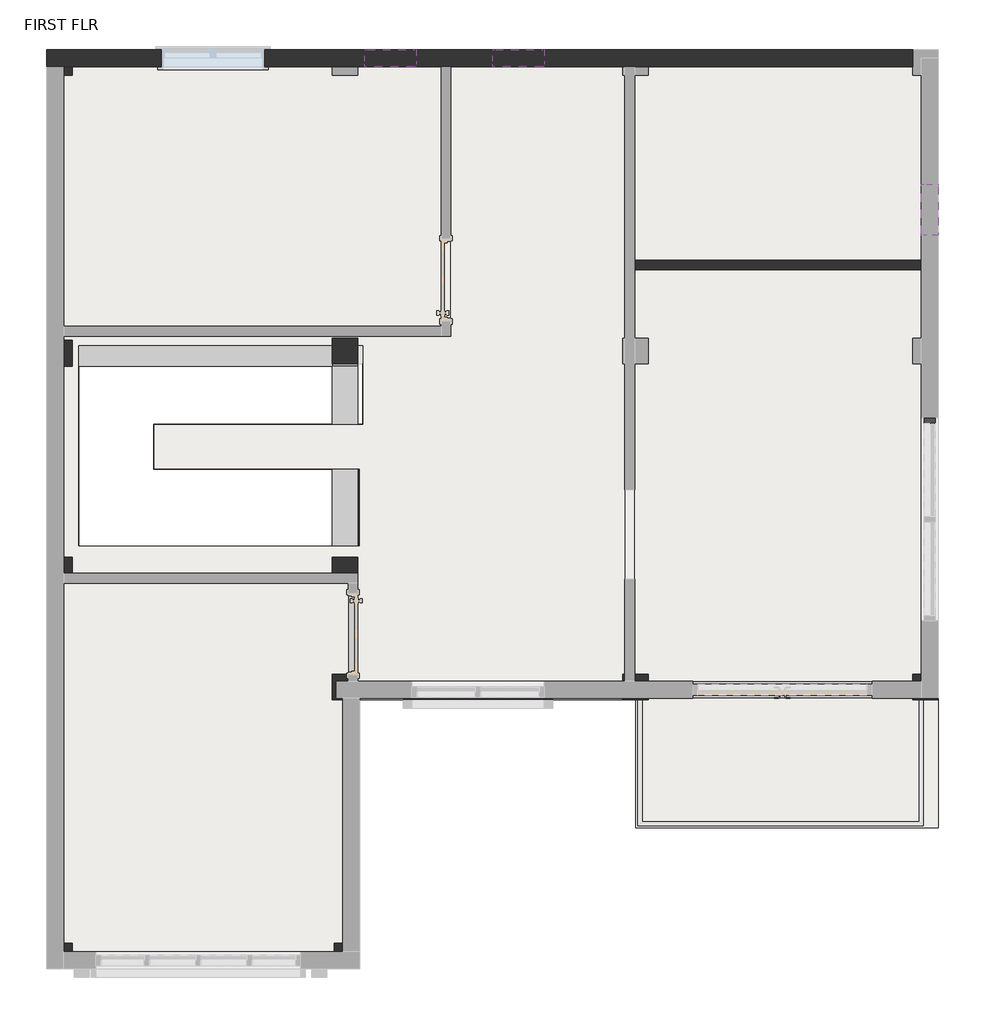
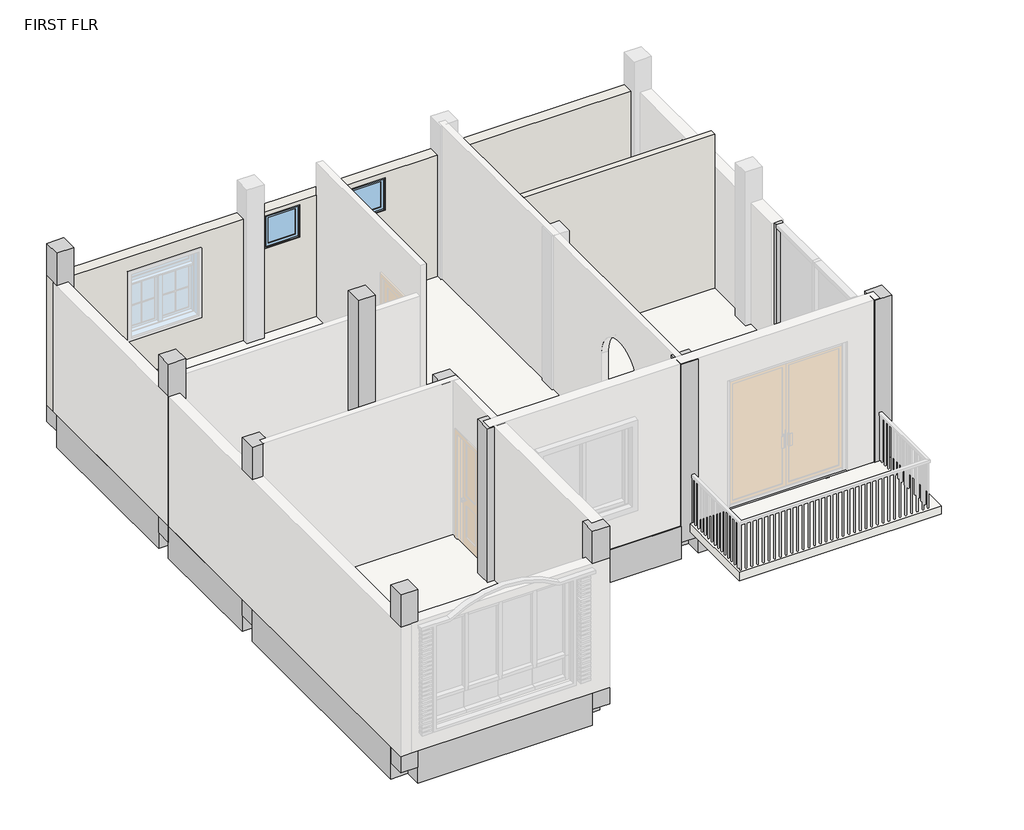
# One storey, part 2 of 3: 15 beams, 10 columns, 9 slabs, 3 windows, 2 walls, 1 member.
"""IFC4 building model written with IfcOpenShell, lengths in millimetres."""

from ifc_helpers import new_model, si_unit, frame, origin, place, context, project, spatial, polyline, outline, extrude, faceted_brep, transform, mapped, element, save
from components import member_5f9244a4, window_6846e476, window_347e55ac

model = new_model("IFC4")

# Units and contexts
model_context = context("Model", 3, world=origin())
ifc_project = project(units=[si_unit("LENGTHUNIT", "METRE", prefix="MILLI")], contexts=[model_context])

# Site, building, storey
site = spatial("IfcSite", under=ifc_project)
building = spatial("IfcBuilding", under=site)
storey = spatial("IfcBuildingStorey", under=building, Name="FIRST FLR", Elevation=3352.8)

# Beams
placement = place(None, origin())
element("IfcBeam", 1, ObjectType="Concrete-Rectangular Beam : 12 x 24", at=placement, inside=storey, context=model_context, shape_type="Brep", body=[
    faceted_brep([(-11643.8293601, -6018.4747117, 3352.8), (-11339.0293601, -6018.4747117, 3352.8), (-11339.0293601, -2868.8747117, 3352.8), (-11643.8293601, -2868.8747117, 3352.8), (-11643.8293601, -6018.4747117, 2743.2), (-11643.8293601, -6018.4747117, 3048.0), (-11643.8293601, -2868.8747117, 3048.0), (-11643.8293601, -2868.8747117, 2743.2), (-11339.0293601, -6018.4747117, 2743.2), (-11339.0293601, -2868.8747117, 2743.2), (-11339.0293601, -6018.4747117, 3048.0), (-11339.0293601, -2868.8747117, 3048.0)], [[[0, 1, 2, 3]], [[4, 5, 0, 3, 6, 7]], [[8, 4, 7, 9]], [[1, 10, 8, 9, 11, 2]], [[2, 11, 9, 7, 6, 3]], [[1, 0, 5, 4, 8, 10]]]),
])
element("IfcBeam", 2, ObjectType="Concrete-Rectangular Beam : 12 x 24", at=placement, inside=storey, context=model_context, shape_type="Brep", body=[
    faceted_brep([(-8251.5270642, -2868.8747117, 3352.8), (-8251.5270642, -2564.0747117, 3352.8), (-11339.0293601, -2564.0747117, 3352.8), (-11339.0293601, -2868.8747117, 3352.8), (-8251.5270642, -2868.8747117, 2743.2), (-8251.5270642, -2868.8747117, 3048.0), (-11339.0293601, -2868.8747117, 3048.0), (-11339.0293601, -2868.8747117, 2743.2), (-8251.5270642, -2564.0747117, 2743.2), (-11339.0293601, -2564.0747117, 2743.2), (-8251.5270642, -2564.0747117, 3048.0), (-11339.0293601, -2564.0747117, 3048.0)], [[[0, 1, 2, 3]], [[4, 5, 0, 3, 6, 7]], [[8, 4, 7, 9]], [[1, 10, 8, 9, 11, 2]], [[2, 11, 9, 7, 6, 3]], [[1, 0, 5, 4, 8, 10]]]),
])
element("IfcBeam", 3, ObjectType="Concrete-Rectangular Beam : 12 x 24", at=placement, inside=storey, context=model_context, shape_type="Brep", body=[
    faceted_brep([(-7946.7270642, -2868.8747117, 3352.8), (-8251.5270642, -2868.8747117, 3352.8), (-8251.5270642, -5993.0747117, 3352.8), (-7946.7270642, -5993.0747117, 3352.8), (-8251.5270642, -2868.8747117, 3048.0), (-8251.5270642, -2868.8747117, 2743.2), (-8251.5270642, -5993.0747117, 2743.2), (-8251.5270642, -5993.0747117, 3048.0), (-7946.7270642, -2868.8747117, 2743.2), (-7946.7270642, -5993.0747117, 2743.2), (-7946.7270642, -2868.8747117, 3048.0), (-7946.7270642, -5993.0747117, 3048.0)], [[[0, 1, 2, 3]], [[1, 4, 5, 6, 7, 2]], [[5, 8, 9, 6]], [[8, 10, 0, 3, 11, 9]], [[0, 10, 8, 5, 4, 1]], [[3, 2, 7, 6, 9, 11]]]),
    faceted_brep([(-7946.7270642, -6323.2747117, 3352.8), (-8251.5270642, -6323.2747117, 3352.8), (-8251.5270642, -6323.2747117, 2743.2), (-7946.7270642, -6323.2747117, 2743.2), (-8251.5270642, -6297.8747117, 3352.8), (-7946.7270642, -6297.8747117, 3352.8), (-7946.7270642, -6297.8747117, 3048.0), (-7946.7270642, -6297.8747117, 2743.2), (-8251.5270642, -6297.8747117, 2743.2), (-8251.5270642, -6297.8747117, 3048.0)], [[[0, 1, 2, 3]], [[4, 5, 6, 7, 8, 9]], [[1, 0, 5, 4]], [[2, 1, 4, 9, 8]], [[3, 2, 8, 7]], [[0, 3, 7, 6, 5]]]),
])
element("IfcBeam", 4, ObjectType="Concrete-Rectangular Beam : 12 x 24", at=placement, inside=storey, context=model_context, shape_type="Brep", body=[
    faceted_brep([(-1351.9658472, -9984.0050402, 3352.8), (-1047.1658472, -9984.0050402, 3352.8), (-1047.1658472, -6297.8747117, 3352.8), (-1351.9658472, -6297.8747117, 3352.8), (-1351.9658472, -9984.0050402, 2743.2), (-1351.9658472, -9984.0050402, 3048.0), (-1351.9658472, -6297.8747117, 3048.0), (-1351.9658472, -6297.8747117, 2743.2), (-1047.1658472, -9984.0050402, 2743.2), (-1047.1658472, -6297.8747117, 2743.2), (-1047.1658472, -9984.0050402, 3048.0), (-1047.1658472, -6297.8747117, 3048.0)], [[[0, 1, 2, 3]], [[4, 5, 0, 3, 6, 7]], [[8, 4, 7, 9]], [[1, 10, 8, 9, 11, 2]], [[2, 11, 9, 7, 6, 3]], [[1, 0, 5, 4, 8, 10]]]),
])
element("IfcBeam", 5, ObjectType="Concrete-Rectangular Beam : 12 x 24", at=placement, inside=storey, context=model_context, shape_type="Brep", body=[
    faceted_brep([(-4492.3270642, -9984.0050402, 3352.8), (-4492.3270642, -10288.8050402, 3352.8), (-1351.9658472, -10288.8050402, 3352.8), (-1351.9658472, -9984.0050402, 3352.8), (-4492.3270642, -9984.0050402, 2743.2), (-4492.3270642, -9984.0050402, 3048.0), (-1351.9658472, -9984.0050402, 3048.0), (-1351.9658472, -9984.0050402, 2743.2), (-4492.3270642, -10288.8050402, 2743.2), (-1351.9658472, -10288.8050402, 2743.2), (-4492.3270642, -10288.8050402, 3048.0), (-1351.9658472, -10288.8050402, 3048.0)], [[[0, 1, 2, 3]], [[4, 5, 0, 3, 6, 7]], [[8, 4, 7, 9]], [[1, 10, 8, 9, 11, 2]], [[1, 0, 5, 4, 8, 10]], [[2, 11, 9, 7, 6, 3]]]),
])
element("IfcBeam", 6, ObjectType="Concrete-Rectangular Beam : 12 x 24", at=placement, inside=storey, context=model_context, shape_type="Brep", body=[
    faceted_brep([(-7946.7270642, -9984.0050402, 3352.8), (-7946.7270642, -10288.8050402, 3352.8), (-7921.3270642, -10288.8050402, 3352.8), (-4797.1270642, -10288.8050402, 3352.8), (-4797.1270642, -9984.0050402, 3352.8), (-4801.7464557, -9984.0050402, 3352.8), (-7942.1076727, -9984.0050402, 3352.8), (-7946.7270642, -9984.0050402, 2743.2), (-7946.7270642, -9984.0050402, 3048.0), (-4797.1270642, -9984.0050402, 3048.0), (-4797.1270642, -9984.0050402, 2743.2), (-7946.7270642, -10288.8050402, 2743.2), (-4797.1270642, -10288.8050402, 2743.2), (-7921.3270642, -10288.8050402, 2743.2), (-7946.7270642, -10288.8050402, 3048.0), (-4797.1270642, -10288.8050402, 3048.0)], [[[0, 1, 2, 3, 4, 5, 6]], [[7, 8, 0, 6, 5, 4, 9, 10]], [[11, 7, 10, 12, 13]], [[1, 14, 11, 13, 12, 15, 3, 2]], [[1, 0, 8, 7, 11, 14]], [[3, 15, 12, 10, 9, 4]]]),
])
element("IfcBeam", 7, ObjectType="Concrete-Rectangular Beam : 12 x 24", at=placement, inside=storey, context=model_context, shape_type="Brep", body=[
    faceted_brep([(-7946.7270642, -9984.0050402, 3352.8), (-7946.7270642, -8902.7373391, 3352.8), (-8226.1270642, -8902.7373391, 3352.8), (-8226.1270642, -9984.0050402, 3352.8), (-7946.7270642, -9984.0050402, 3048.0), (-7946.7270642, -9984.0050402, 2743.2), (-7946.7270642, -8902.7373391, 2743.2), (-7946.7270642, -8902.7373391, 3048.0), (-8251.5270642, -9984.0050402, 2743.2), (-8251.5270642, -8902.7373391, 2743.2), (-8251.5270642, -9984.0050402, 3048.0), (-8251.5270642, -8902.7373391, 3048.0), (-8226.1270642, -8902.7373391, 3048.0), (-8226.1270642, -9984.0050402, 3048.0)], [[[0, 1, 2, 3]], [[1, 0, 4, 5, 6, 7]], [[6, 5, 8, 9]], [[9, 8, 10, 11]], [[1, 7, 6, 9, 11, 12, 2]], [[8, 5, 4, 0, 3, 13, 10]], [[13, 12, 11, 10]], [[12, 13, 3, 2]]]),
])
element("IfcBeam", 8, ObjectType="Concrete-Rectangular Beam : 12 x 24", at=placement, inside=storey, context=model_context, shape_type="Brep", body=[
    faceted_brep([(-8251.5270642, -8597.9373391, 3352.8), (-7946.7270642, -8597.9373391, 3352.8), (-7946.7270642, -6323.2747117, 3352.8), (-8251.5270642, -6323.2747117, 3352.8), (-8251.5270642, -7013.8396616, 3352.8), (-8251.5270642, -7547.2396616, 3352.8), (-8251.5270642, -8461.6396616, 3352.8), (-7946.7270642, -8597.9373391, 3048.0), (-7946.7270642, -8597.9373391, 2743.2), (-7946.7270642, -6323.2747117, 2743.2), (-8251.5270642, -8597.9373391, 2743.2), (-8251.5270642, -6323.2747117, 2743.2), (-8251.5270642, -8597.9373391, 3048.0)], [[[0, 1, 2, 3, 4, 5, 6]], [[1, 7, 8, 9, 2]], [[8, 10, 11, 9]], [[10, 12, 0, 6, 5, 4, 3, 11]], [[0, 12, 10, 8, 7, 1]], [[3, 2, 9, 11]]]),
])
element("IfcBeam", 9, ObjectType="Concrete-Rectangular Beam : 12 x 24", at=placement, inside=storey, context=model_context, shape_type="Brep", body=[
    faceted_brep([(-11339.0293601, -8597.9373391, 3352.8), (-11339.0293601, -8902.7373391, 3352.8), (-8251.5270642, -8902.7373391, 3352.8), (-8251.5270642, -8597.9373391, 3352.8), (-11339.0293601, -8597.9373391, 2743.2), (-11339.0293601, -8597.9373391, 3048.0), (-8251.5270642, -8597.9373391, 3048.0), (-8251.5270642, -8597.9373391, 2743.2), (-11339.0293601, -8902.7373391, 2743.2), (-8251.5270642, -8902.7373391, 2743.2), (-11339.0293601, -8902.7373391, 3048.0), (-8251.5270642, -8902.7373391, 3048.0)], [[[0, 1, 2, 3]], [[4, 5, 0, 3, 6, 7]], [[8, 4, 7, 9]], [[1, 10, 8, 9, 11, 2]], [[1, 0, 5, 4, 8, 10]], [[2, 11, 9, 7, 6, 3]]]),
])
element("IfcBeam", 10, ObjectType="Concrete-Rectangular Beam : 12 x 24", at=placement, inside=storey, context=model_context, shape_type="Brep", body=[
    faceted_brep([(-11339.0293601, -6323.2747117, 3352.8), (-11643.8293601, -6323.2747117, 3352.8), (-11643.8293601, -8597.9373391, 3352.8), (-11339.0293601, -8597.9373391, 3352.8), (-11339.0293601, -6323.2747117, 2743.2), (-11339.0293601, -6323.2747117, 3048.0), (-11339.0293601, -8597.9373391, 3048.0), (-11339.0293601, -8597.9373391, 2743.2), (-11643.8293601, -6323.2747117, 2743.2), (-11643.8293601, -8597.9373391, 2743.2), (-11643.8293601, -6323.2747117, 3048.0), (-11643.8293601, -8597.9373391, 3048.0)], [[[0, 1, 2, 3]], [[4, 5, 0, 3, 6, 7]], [[8, 4, 7, 9]], [[1, 10, 8, 9, 11, 2]], [[1, 0, 5, 4, 8, 10]], [[2, 11, 9, 7, 6, 3]]]),
])
element("IfcBeam", 11, ObjectType="Concrete-Rectangular Beam : 12 x 24", at=placement, inside=storey, context=model_context, shape_type="Brep", body=[
    faceted_brep([(-8251.5270642, -6018.4747117, 3352.8), (-8251.5270642, -6297.8747117, 3352.8), (-8251.5270642, -6323.2747117, 3352.8), (-8251.5270642, -6323.2747117, 2743.2), (-8251.5270642, -6297.8747117, 2743.2), (-8251.5270642, -6018.4747117, 2743.2), (-8251.5270642, -6018.4747117, 3048.0), (-11339.0293601, -6018.4747117, 3352.8), (-11339.0293601, -6323.2747117, 3352.8), (-11264.7236584, -6323.2747117, 3352.8), (-11339.0293601, -6323.2747117, 3048.0), (-11339.0293601, -6323.2747117, 2743.2), (-11339.0293601, -6018.4747117, 2743.2), (-11339.0293601, -6018.4747117, 3048.0)], [[[0, 1, 2, 3, 4, 5, 6]], [[2, 1, 0, 7, 8, 9]], [[3, 2, 9, 8, 10, 11]], [[5, 4, 3, 11, 12]], [[0, 6, 5, 12, 13, 7]], [[7, 13, 12, 11, 10, 8]]]),
])
element("IfcBeam", 12, ObjectType="Concrete-Rectangular Beam : 12 x 24", at=placement, inside=storey, context=model_context, shape_type="Brep", body=[
    faceted_brep([(-4492.3270642, -6297.8747117, 3352.8), (-4797.1270642, -6297.8747117, 3352.8), (-4797.1270642, -9984.0050402, 3352.8), (-4492.3270642, -9984.0050402, 3352.8), (-4492.3270642, -6297.8747117, 2743.2), (-4492.3270642, -6297.8747117, 3048.0), (-4492.3270642, -9984.0050402, 3048.0), (-4492.3270642, -9984.0050402, 2743.2), (-4797.1270642, -6297.8747117, 2743.2), (-4797.1270642, -9984.0050402, 2743.2), (-4797.1270642, -6297.8747117, 3048.0), (-4797.1270642, -9984.0050402, 3048.0)], [[[0, 1, 2, 3]], [[4, 5, 0, 3, 6, 7]], [[8, 4, 7, 9]], [[1, 10, 8, 9, 11, 2]], [[1, 0, 5, 4, 8, 10]], [[2, 11, 9, 7, 6, 3]]]),
])
element("IfcBeam", 13, ObjectType="Concrete-Rectangular Beam : 12 x 24", at=placement, inside=storey, context=model_context, shape_type="Brep", body=[
    faceted_brep([(-11339.0293601, -8902.7373391, 3352.8), (-11643.8293601, -8902.7373391, 3352.8), (-11643.8293601, -13183.002305, 3352.8), (-11339.0293601, -13183.002305, 3352.8), (-11339.0293601, -8902.7373391, 2743.2), (-11339.0293601, -8902.7373391, 3048.0), (-11339.0293601, -13183.002305, 3048.0), (-11339.0293601, -13183.002305, 2743.2), (-11643.8293601, -8902.7373391, 2743.2), (-11643.8293601, -13183.002305, 2743.2), (-11643.8293601, -8902.7373391, 3048.0), (-11643.8293601, -13183.002305, 3048.0)], [[[0, 1, 2, 3]], [[4, 5, 0, 3, 6, 7]], [[8, 4, 7, 9]], [[1, 10, 8, 9, 11, 2]], [[1, 0, 5, 4, 8, 10]], [[2, 11, 9, 7, 6, 3]]]),
])
element("IfcBeam", 14, ObjectType="Concrete-Rectangular Beam : 12 x 24", at=placement, inside=storey, context=model_context, shape_type="Brep", body=[
    faceted_brep([(-7921.3270642, -10288.8050402, 3352.8), (-7946.7270642, -10288.8050402, 3352.8), (-8226.1270642, -10288.8050402, 3352.8), (-8226.1270642, -13183.002305, 3352.8), (-7921.3270642, -13183.002305, 3352.8), (-8226.1270642, -10288.8050402, 3048.0), (-8226.1270642, -10288.8050402, 2743.2), (-8226.1270642, -13183.002305, 2743.2), (-8226.1270642, -13183.002305, 3048.0), (-7946.7270642, -10288.8050402, 2743.2), (-7921.3270642, -10288.8050402, 2743.2), (-7921.3270642, -13183.002305, 2743.2), (-7921.3270642, -13183.002305, 3048.0)], [[[0, 1, 2, 3, 4]], [[2, 5, 6, 7, 8, 3]], [[6, 9, 10, 11, 7]], [[10, 0, 4, 12, 11]], [[0, 10, 9, 6, 5, 2, 1]], [[4, 3, 8, 7, 11, 12]]]),
])
element("IfcBeam", 15, ObjectType="Concrete-Rectangular Beam : 12 x 24", at=placement, inside=storey, context=model_context, shape_type="Brep", body=[
    faceted_brep([(-11339.0293601, -13183.002305, 3352.8), (-11339.0293601, -13487.802305, 3352.8), (-8226.1270642, -13487.802305, 3352.8), (-8226.1270642, -13183.002305, 3352.8), (-11339.0293601, -13183.002305, 2743.2), (-11339.0293601, -13183.002305, 3048.0), (-8226.1270642, -13183.002305, 3048.0), (-8226.1270642, -13183.002305, 2743.2), (-11339.0293601, -13487.802305, 2743.2), (-8226.1270642, -13487.802305, 2743.2), (-11339.0293601, -13487.802305, 3048.0), (-8226.1270642, -13487.802305, 3048.0)], [[[0, 1, 2, 3]], [[4, 5, 0, 3, 6, 7]], [[8, 4, 7, 9]], [[1, 10, 8, 9, 11, 2]], [[2, 11, 9, 7, 6, 3]], [[1, 0, 5, 4, 8, 10]]]),
])

# Columns
element("IfcColumn", 16, ObjectType="Concrete-Rectangular-Column : 12\" X 12\" COLUMN", at=placement, inside=storey, context=model_context, shape_type="Brep", body=[
    faceted_brep([(-11339.0293601, -2564.0747117, 3048.0), (-11339.0293601, -2868.8747117, 3048.0), (-11643.8293601, -2868.8747117, 3048.0), (-11643.8293601, -2564.0747117, 3048.0), (-11339.0293601, -2564.0747117, 6400.8), (-11339.0293601, -2868.8747117, 6400.8), (-11339.0293601, -2868.8747117, 3352.8), (-11339.0293601, -2564.0747117, 3352.8), (-11643.8293601, -2868.8747117, 6400.8), (-11643.8293601, -2868.8747117, 3352.8), (-11643.8293601, -2564.0747117, 6400.8)], [[[0, 1, 2, 3]], [[4, 5, 6, 1, 0, 7]], [[5, 8, 9, 2, 1, 6]], [[8, 10, 3, 2, 9]], [[10, 4, 7, 0, 3]], [[4, 10, 8, 5]]]),
])
element("IfcColumn", 17, ObjectType="Concrete-Rectangular-Column : 12\" X 12\" COLUMN", at=placement, inside=storey, context=model_context, shape_type="Brep", body=[
    faceted_brep([(-7946.7270642, -5993.0747117, 3048.0), (-7946.7270642, -6297.8747117, 3048.0), (-8251.5270642, -6297.8747117, 3048.0), (-8251.5270642, -6018.4747117, 3048.0), (-8251.5270642, -5993.0747117, 3048.0), (-7946.7270642, -5993.0747117, 6400.8), (-7946.7270642, -6297.8747117, 6400.8), (-7946.7270642, -6297.8747117, 3352.8), (-7946.7270642, -5993.0747117, 3352.8), (-8251.5270642, -6297.8747117, 6400.8), (-8251.5270642, -6297.8747117, 3352.8), (-8251.5270642, -5993.0747117, 6400.8), (-8251.5270642, -5993.0747117, 3352.8)], [[[0, 1, 2, 3, 4]], [[5, 6, 7, 1, 0, 8]], [[6, 9, 10, 2, 1, 7]], [[9, 11, 12, 4, 3, 2, 10]], [[11, 5, 8, 0, 4, 12]], [[5, 11, 9, 6]]]),
])
element("IfcColumn", 18, ObjectType="Concrete-Rectangular-Column : 12\" X 12\" COLUMN", at=placement, inside=storey, context=model_context, shape_type="Brep", body=[
    faceted_brep([(-11339.0293601, -6018.4747117, 3048.0), (-11339.0293601, -6323.2747117, 3048.0), (-11643.8293601, -6323.2747117, 3048.0), (-11643.8293601, -6018.4747117, 3048.0), (-11339.0293601, -6018.4747117, 6400.8), (-11339.0293601, -6323.2747117, 6400.8), (-11339.0293601, -6323.2747117, 3352.8), (-11339.0293601, -6018.4747117, 3352.8), (-11643.8293601, -6323.2747117, 6400.8), (-11643.8293601, -6323.2747117, 3352.8), (-11643.8293601, -6018.4747117, 6400.8), (-11643.8293601, -6018.4747117, 3352.8)], [[[0, 1, 2, 3]], [[4, 5, 6, 1, 0, 7]], [[5, 8, 9, 2, 1, 6]], [[8, 10, 11, 3, 2, 9]], [[10, 4, 7, 0, 3, 11]], [[4, 10, 8, 5]]]),
])
element("IfcColumn", 19, ObjectType="Concrete-Rectangular-Column : 12\" X 12\" COLUMN", at=placement, inside=storey, context=model_context, shape_type="Brep", body=[
    faceted_brep([(-11339.0293601, -8597.9373391, 3048.0), (-11339.0293601, -8902.7373391, 3048.0), (-11643.8293601, -8902.7373391, 3048.0), (-11643.8293601, -8597.9373391, 3048.0), (-11339.0293601, -8597.9373391, 6400.8), (-11339.0293601, -8902.7373391, 6400.8), (-11339.0293601, -8902.7373391, 3352.8), (-11339.0293601, -8597.9373391, 3352.8), (-11643.8293601, -8902.7373391, 6400.8), (-11643.8293601, -8902.7373391, 3352.8), (-11643.8293601, -8597.9373391, 6400.8), (-11643.8293601, -8597.9373391, 3352.8)], [[[0, 1, 2, 3]], [[4, 5, 6, 1, 0, 7]], [[5, 8, 9, 2, 1, 6]], [[8, 10, 11, 3, 2, 9]], [[10, 4, 7, 0, 3, 11]], [[4, 10, 8, 5]]]),
])
element("IfcColumn", 20, ObjectType="Concrete-Rectangular-Column : 12\" X 12\" COLUMN", at=placement, inside=storey, context=model_context, shape_type="Brep", body=[
    faceted_brep([(-7946.7270642, -8597.9373391, 3048.0), (-7946.7270642, -8902.7373391, 3048.0), (-8251.5270642, -8902.7373391, 3048.0), (-8251.5270642, -8597.9373391, 3048.0), (-7946.7270642, -8597.9373391, 6400.8), (-7946.7270642, -8902.7373391, 6400.8), (-7946.7270642, -8902.7373391, 3352.8), (-7946.7270642, -8597.9373391, 3352.8), (-8251.5270642, -8902.7373391, 6400.8), (-8251.5270642, -8902.7373391, 3352.8), (-8251.5270642, -8597.9373391, 6400.8), (-8251.5270642, -8597.9373391, 3352.8)], [[[0, 1, 2, 3]], [[4, 5, 6, 1, 0, 7]], [[5, 8, 9, 2, 1, 6]], [[8, 10, 11, 3, 2, 9]], [[10, 4, 7, 0, 3, 11]], [[4, 10, 8, 5]]]),
])
element("IfcColumn", 21, ObjectType="Concrete-Rectangular-Column : 12\" X 12\" COLUMN", at=placement, inside=storey, context=model_context, shape_type="Brep", body=[
    faceted_brep([(-7921.3270642, -13183.002305, 3048.0), (-7921.3270642, -13487.802305, 3048.0), (-8226.1270642, -13487.802305, 3048.0), (-8226.1270642, -13183.002305, 3048.0), (-7921.3270642, -13183.002305, 6400.8), (-7921.3270642, -13487.802305, 6400.8), (-7921.3270642, -13183.002305, 3352.8), (-8226.1270642, -13487.802305, 6400.8), (-8226.1270642, -13487.802305, 3352.8), (-8226.1270642, -13183.002305, 6400.8), (-8226.1270642, -13183.002305, 3352.8)], [[[0, 1, 2, 3]], [[4, 5, 1, 0, 6]], [[5, 7, 8, 2, 1]], [[7, 9, 10, 3, 2, 8]], [[9, 4, 6, 0, 3, 10]], [[4, 9, 7, 5]]]),
])
element("IfcColumn", 22, ObjectType="Concrete-Rectangular-Column : 12\" X 12\" COLUMN", at=placement, inside=storey, context=model_context, shape_type="Brep", body=[
    faceted_brep([(-11339.0293601, -13183.002305, 3048.0), (-11339.0293601, -13487.802305, 3048.0), (-11643.8293601, -13487.802305, 3048.0), (-11643.8293601, -13183.002305, 3048.0), (-11339.0293601, -13183.002305, 6400.8), (-11339.0293601, -13487.802305, 6400.8), (-11339.0293601, -13487.802305, 3352.8), (-11339.0293601, -13183.002305, 3352.8), (-11643.8293601, -13487.802305, 6400.8), (-11643.8293601, -13183.002305, 6400.8), (-11643.8293601, -13183.002305, 3352.8)], [[[0, 1, 2, 3]], [[4, 5, 6, 1, 0, 7]], [[5, 8, 2, 1, 6]], [[8, 9, 10, 3, 2]], [[9, 4, 7, 0, 3, 10]], [[4, 9, 8, 5]]]),
])
element("IfcColumn", 23, ObjectType="Concrete-Rectangular-Column : 12\" X 12\" COLUMN", at=placement, inside=storey, context=model_context, shape_type="Brep", body=[
    faceted_brep([(-7946.7270642, -9984.0050402, 3048.0), (-7946.7270642, -10288.8050402, 3048.0), (-8226.1270642, -10288.8050402, 3048.0), (-8226.1270642, -9984.0050402, 3048.0), (-7946.7270642, -9984.0050402, 3352.8), (-7946.7270642, -9984.0050402, 6400.8), (-7946.7270642, -10288.8050402, 6400.8), (-7946.7270642, -10288.8050402, 3352.8), (-8251.5270642, -10288.8050402, 6400.8), (-8251.5270642, -10288.8050402, 3352.8), (-8226.1270642, -10288.8050402, 3352.8), (-8251.5270642, -9984.0050402, 6400.8), (-8251.5270642, -9984.0050402, 3352.8), (-8226.1270642, -9984.0050402, 3352.8)], [[[0, 1, 2, 3]], [[1, 0, 4, 5, 6, 7]], [[1, 7, 6, 8, 9, 10, 2]], [[8, 11, 12, 9]], [[5, 4, 0, 3, 13, 12, 11]], [[6, 5, 11, 8]], [[13, 10, 9, 12]], [[10, 13, 3, 2]]]),
])
element("IfcColumn", 24, ObjectType="Concrete-Rectangular-Column : 12\" X 12\" COLUMN", at=placement, inside=storey, context=model_context, shape_type="Brep", body=[
    faceted_brep([(-4492.3270642, -9984.0050402, 3048.0), (-4492.3270642, -10288.8050402, 3048.0), (-4797.1270642, -10288.8050402, 3048.0), (-4797.1270642, -9984.0050402, 3048.0), (-4492.3270642, -9984.0050402, 6400.8), (-4492.3270642, -10288.8050402, 6400.8), (-4492.3270642, -10288.8050402, 3352.8), (-4492.3270642, -9984.0050402, 3352.8), (-4797.1270642, -10288.8050402, 6400.8), (-4797.1270642, -10288.8050402, 3352.8), (-4797.1270642, -9984.0050402, 6400.8), (-4797.1270642, -9984.0050402, 3352.8)], [[[0, 1, 2, 3]], [[4, 5, 6, 1, 0, 7]], [[5, 8, 9, 2, 1, 6]], [[8, 10, 11, 3, 2, 9]], [[10, 4, 7, 0, 3, 11]], [[4, 10, 8, 5]]]),
])
element("IfcColumn", 25, ObjectType="Concrete-Rectangular-Column : 12\" X 12\" COLUMN", at=placement, inside=storey, context=model_context, shape_type="Brep", body=[
    faceted_brep([(-1047.1658472, -9984.0050402, 3048.0), (-1047.1658472, -10288.8050402, 3048.0), (-1351.9658472, -10288.8050402, 3048.0), (-1351.9658472, -9984.0050402, 3048.0), (-1047.1658472, -9984.0050402, 6400.8), (-1047.1658472, -10288.8050402, 6400.8), (-1047.1658472, -9984.0050402, 3352.8), (-1351.9658472, -10288.8050402, 6400.8), (-1351.9658472, -10288.8050402, 3352.8), (-1351.9658472, -9984.0050402, 6400.8), (-1351.9658472, -9984.0050402, 3352.8)], [[[0, 1, 2, 3]], [[4, 5, 1, 0, 6]], [[5, 7, 8, 2, 1]], [[7, 9, 10, 3, 2, 8]], [[9, 4, 6, 0, 3, 10]], [[4, 9, 7, 5]]]),
])

# Member
member_shape = member_5f9244a4(model_context)
element("IfcMember", 26, ObjectType="Rectangular Mullion : 2.5\" x 5\" rectangular", at=placement, inside=storey, context=model_context, shape_type="MappedRepresentation", body=[
    mapped(member_shape, transform((-1148.7658472, -6939.2247117, 5791.2), x_axis=(0.0, 1.0, 0.0), y_axis=(-1.0, 0.0, 0.0), z_axis=(0.0, 0.0, 1.0))),
])

# Slabs
element("IfcSlab", 27, ObjectType="FLOORING 6\"", at=placement, inside=storey, context=model_context, shape_type="SweptSolid", body=[
    extrude(outline(polyline([(-4644.7270642, -10271.3896616), (-1047.1658472, -10271.3896616), (-1047.1658472, -11812.34549), (-4644.7270642, -11812.34549), (-4644.7270642, -10271.3896616)])), frame((0.0, 0.0, 3200.4), z_axis=(0.0, 0.0, 1.0), x_axis=(1.0, 0.0, 0.0)), (0.0, 0.0, 1.0), 152.4),
])
element("IfcSlab", 28, ObjectType="FLOORING 6\"", at=placement, inside=storey, context=model_context, shape_type="SweptSolid", body=[
    extrude(outline(polyline([(-6956.1270642, -2767.2747117), (-6956.1270642, -5851.7896616), (-11442.5236584, -5851.7896616), (-11442.5236584, -2767.2747117), (-6956.1270642, -2767.2747117)])), frame((0.0, 0.0, 3352.8), z_axis=(0.0, 0.0, 1.0), x_axis=(1.0, 0.0, 0.0)), (0.0, 0.0, 1.0), 152.4),
    extrude(outline(polyline([(-1250.3658472, -2767.2747117), (-1250.3658472, -5064.3896616), (-4657.4270642, -5064.3896616), (-4657.4270642, -2767.2747117), (-1250.3658472, -2767.2747117)])), frame((0.0, 0.0, 3352.8), z_axis=(0.0, 0.0, 1.0), x_axis=(1.0, 0.0, 0.0)), (0.0, 0.0, 1.0), 152.4),
    extrude(outline(polyline([(-4657.4270642, -10068.1896616), (-4657.4270642, -5178.6896616), (-1250.3658472, -5178.6896616), (-1250.3658472, -10068.1896616), (-4657.4270642, -10068.1896616)])), frame((0.0, 0.0, 3352.8), z_axis=(0.0, 0.0, 1.0), x_axis=(1.0, 0.0, 0.0)), (0.0, 0.0, 1.0), 152.4),
    extrude(outline(polyline([(-8061.0270642, -8902.7373391), (-8061.0270642, -10068.1896616), (-8200.7270642, -10068.1896616), (-8200.7270642, -10271.3896616), (-8124.5270642, -10271.3896616), (-8124.5270642, -13284.602305), (-11442.5236584, -13284.602305), (-11442.5236584, -8902.7373391), (-8061.0270642, -8902.7373391)])), frame((0.0, 0.0, 3352.8), z_axis=(0.0, 0.0, 1.0), x_axis=(1.0, 0.0, 0.0)), (0.0, 0.0, 1.0), 152.4),
    extrude(outline(polyline([(-6841.8270642, -5966.0896616), (-6841.8270642, -2767.2747117), (-4771.7270642, -2767.2747117), (-4771.7270642, -10068.1896616), (-7946.7270642, -10068.1896616), (-7946.7270642, -8788.4373391), (-11442.5236584, -8788.4373391), (-11442.5236584, -5966.0896616), (-6841.8270642, -5966.0896616)]), holes=[polyline([(-11264.7236584, -6080.3896616), (-11264.7236584, -8461.6396616), (-7930.9736584, -8461.6396616), (-7930.9736584, -7547.2396616), (-10369.3736584, -7547.2396616), (-10369.3736584, -7013.8396616), (-7889.5770642, -7013.8396616), (-7889.5770642, -6080.3896616), (-11264.7236584, -6080.3896616)])]), frame((0.0, 0.0, 3352.8), z_axis=(0.0, 0.0, 1.0), x_axis=(1.0, 0.0, 0.0)), (0.0, 0.0, 1.0), 152.4),
])
element("IfcSlab", 29, ObjectType="Generic - 12\"", at=placement, inside=storey, context=model_context, shape_type="Brep", body=[
    faceted_brep([(-8251.5270642, -2868.8747117, 3048.0), (-8251.5270642, -5993.0747117, 3048.0), (-8251.5270642, -6018.4747117, 3048.0), (-11339.0293601, -6018.4747117, 3048.0), (-11339.0293601, -2868.8747117, 3048.0), (-8251.5270642, -2868.8747117, 3352.8), (-11339.0293601, -2868.8747117, 3352.8), (-11339.0293601, -6018.4747117, 3352.8), (-8251.5270642, -6018.4747117, 3352.8), (-8251.5270642, -5993.0747117, 3352.8)], [[[0, 1, 2, 3, 4]], [[5, 6, 7, 8, 9]], [[2, 1, 0, 5, 9, 8]], [[3, 2, 8, 7]], [[4, 3, 7, 6]], [[0, 4, 6, 5]]]),
])
element("IfcSlab", 30, ObjectType="Generic - 12\"", at=placement, inside=storey, context=model_context, shape_type="SweptSolid", body=[
    extrude(outline(polyline([(-4797.1270642, -2868.8747117), (-4797.1270642, -5993.0747117), (-7946.7270642, -5993.0747117), (-7946.7270642, -2868.8747117), (-4797.1270642, -2868.8747117)])), frame((0.0, 0.0, 3048.0), z_axis=(0.0, 0.0, 1.0), x_axis=(1.0, 0.0, 0.0)), (0.0, 0.0, 1.0), 304.8),
])
element("IfcSlab", 31, ObjectType="Generic - 12\"", at=placement, inside=storey, context=model_context, shape_type="SweptSolid", body=[
    extrude(outline(polyline([(-1351.9658472, -2868.8747117), (-1351.9658472, -5993.0747117), (-4492.3270642, -5993.0747117), (-4492.3270642, -2868.8747117), (-1351.9658472, -2868.8747117)])), frame((0.0, 0.0, 3048.0), z_axis=(0.0, 0.0, 1.0), x_axis=(1.0, 0.0, 0.0)), (0.0, 0.0, 1.0), 304.8),
])
element("IfcSlab", 32, ObjectType="Generic - 12\"", at=placement, inside=storey, context=model_context, shape_type="SweptSolid", body=[
    extrude(outline(polyline([(-1351.9658472, -6297.8747117), (-1351.9658472, -9984.0050402), (-4492.3270642, -9984.0050402), (-4492.3270642, -6297.8747117), (-1351.9658472, -6297.8747117)])), frame((0.0, 0.0, 3048.0), z_axis=(0.0, 0.0, 1.0), x_axis=(1.0, 0.0, 0.0)), (0.0, 0.0, 1.0), 304.8),
])
element("IfcSlab", 33, ObjectType="Generic - 12\"", at=placement, inside=storey, context=model_context, shape_type="SweptSolid", body=[
    extrude(outline(polyline([(-4801.7464557, -6297.8747117), (-4801.7464557, -9984.0050402), (-7942.1076727, -9984.0050402), (-7942.1076727, -8461.6396616), (-7930.9736584, -8461.6396616), (-7930.9736584, -7547.2396616), (-7942.1076727, -7547.2396616), (-7942.1076727, -7013.8396616), (-7889.5770642, -7013.8396616), (-7889.5770642, -6297.8747117), (-4801.7464557, -6297.8747117)])), frame((0.0, 0.0, 3048.0), z_axis=(0.0, 0.0, 1.0), x_axis=(1.0, 0.0, 0.0)), (0.0, 0.0, 1.0), 304.8),
])
element("IfcSlab", 34, ObjectType="Generic - 12\"", at=placement, inside=storey, context=model_context, shape_type="SweptSolid", body=[
    extrude(outline(polyline([(-8251.6377222, -8597.9373391), (-11339.0293601, -8597.9373391), (-11339.0293601, -6323.2747117), (-11264.7236584, -6323.2747117), (-11264.7236584, -8461.6396616), (-8251.6377222, -8461.6396616), (-8251.6377222, -8597.9373391)])), frame((0.0, 0.0, 3048.0), z_axis=(0.0, 0.0, 1.0), x_axis=(1.0, 0.0, 0.0)), (0.0, 0.0, 1.0), 304.8),
    extrude(outline(polyline([(-8251.6377222, -7013.8396616), (-8251.6377222, -7547.2396616), (-10369.3736584, -7547.2396616), (-10369.3736584, -7013.8396616), (-8251.6377222, -7013.8396616)])), frame((0.0, 0.0, 3048.0), z_axis=(0.0, 0.0, 1.0), x_axis=(1.0, 0.0, 0.0)), (0.0, 0.0, 1.0), 304.8),
])
element("IfcSlab", 35, ObjectType="Generic - 12\"", at=placement, inside=storey, context=model_context, shape_type="Brep", body=[
    faceted_brep([(-8226.1270642, -8902.7191027, 3048.0), (-8226.1270642, -9984.0050402, 3048.0), (-8226.1270642, -10288.8050402, 3048.0), (-8226.1270642, -13183.002305, 3048.0), (-11339.0293601, -13183.002305, 3048.0), (-11339.0293601, -8902.7191027, 3048.0), (-8226.1270642, -8902.7191027, 3352.8), (-8251.5270642, -8902.7191027, 3352.8), (-11339.0293601, -8902.7191027, 3352.8), (-11339.0293601, -13183.002305, 3352.8), (-8226.1270642, -13183.002305, 3352.8), (-8226.1270642, -10288.8050402, 3352.8), (-8226.1270642, -9984.0050402, 3352.8)], [[[0, 1, 2, 3, 4, 5]], [[6, 7, 8, 9, 10, 11, 12]], [[3, 2, 1, 0, 6, 12, 11, 10]], [[4, 3, 10, 9]], [[5, 4, 9, 8]], [[0, 5, 8, 7, 6]]]),
])

# Walls
element("IfcWall", 36, ObjectType="EXTERIOR 8'", at=placement, inside=storey, context=model_context, shape_type="Brep", body=[
    faceted_brep([(-11645.7236584, -2767.2747117, 3352.8), (-11442.5236584, -2767.2747117, 3352.8), (-6956.1270642, -2767.2747117, 3352.8), (-6841.8270642, -2767.2747117, 3352.8), (-4771.7270642, -2767.2747117, 3352.8), (-4657.4270642, -2767.2747117, 3352.8), (-1351.9658472, -2767.2747117, 3352.8), (-1351.9658472, -2767.2747117, 5791.2), (-11645.7236584, -2767.2747117, 5791.2), (-11645.7236584, -2767.2747117, 5787.4119669), (-9057.9770642, -2767.2747117, 5486.4), (-9057.9770642, -2767.2747117, 4267.2), (-10277.1770642, -2767.2747117, 4267.2), (-10277.1770642, -2767.2747117, 5486.4), (-7864.1770642, -2767.2747117, 5715.0), (-7254.5770642, -2767.2747117, 5715.0), (-7254.5770642, -2767.2747117, 5105.4), (-7864.1770642, -2767.2747117, 5105.4), (-6340.1770642, -2767.2747117, 5689.6), (-5730.5770642, -2767.2747117, 5689.6), (-5730.5770642, -2767.2747117, 5080.0), (-6340.1770642, -2767.2747117, 5080.0), (-11645.7236584, -2564.0747117, 3352.8), (-11645.7236584, -2564.0747117, 5791.2), (-1351.9658472, -2564.0747117, 5791.2), (-1351.9658472, -2564.0747117, 3352.8), (-9057.9770642, -2564.0747117, 5486.4), (-10277.1770642, -2564.0747117, 5486.4), (-10277.1770642, -2564.0747117, 4267.2), (-9057.9770642, -2564.0747117, 4267.2), (-7864.1770642, -2564.0747117, 5715.0), (-7864.1770642, -2564.0747117, 5105.4), (-7254.5770642, -2564.0747117, 5105.4), (-7254.5770642, -2564.0747117, 5715.0), (-6340.1770642, -2564.0747117, 5689.6), (-6340.1770642, -2564.0747117, 5080.0), (-5730.5770642, -2564.0747117, 5080.0), (-5730.5770642, -2564.0747117, 5689.6)], [[[0, 1, 2, 3, 4, 5, 6, 7, 8, 9], [10, 11, 12, 13], [14, 15, 16, 17], [18, 19, 20, 21]], [[22, 23, 24, 25], [26, 27, 28, 29], [30, 31, 32, 33], [34, 35, 36, 37]], [[6, 5, 4, 3, 2, 1, 0, 22, 25]], [[7, 6, 25, 24]], [[8, 7, 24, 23]], [[0, 9, 8, 23, 22]], [[11, 10, 26, 29]], [[12, 11, 29, 28]], [[13, 12, 28, 27]], [[10, 13, 27, 26]], [[31, 30, 14, 17]], [[32, 31, 17, 16]], [[33, 32, 16, 15]], [[30, 33, 15, 14]], [[35, 34, 18, 21]], [[36, 35, 21, 20]], [[37, 36, 20, 19]], [[34, 37, 19, 18]]]),
])
element("IfcWall", 37, ObjectType="interior wall 4.5\"", at=placement, inside=storey, context=model_context, shape_type="SweptSolid", body=[
    extrude(outline(polyline([(-1250.3658472, -5178.6896616), (-4657.4270642, -5178.6896616), (-4657.4270642, -5064.3896616), (-1250.3658472, -5064.3896616), (-1250.3658472, -5178.6896616)])), frame((0.0, 0.0, 3352.8), z_axis=(0.0, 0.0, 1.0), x_axis=(1.0, 0.0, 0.0)), (0.0, 0.0, 1.0), 3048.0),
])

# Windows
window_shape = window_6846e476(model_context)
element("IfcWindow", 38, ObjectType="Fixed : 24\" x 24\"", at=placement, inside=storey, context=model_context, shape_type="MappedRepresentation", body=[
    mapped(window_shape, transform((-6073.4770642, -2665.6747117, 4165.6), x_axis=(-1.0, 0.0, 0.0), y_axis=(0.0, -1.0, 0.0), z_axis=(0.0, 0.0, 1.0))),
])
element("IfcWindow", 39, ObjectType="Fixed : 24\" x 24\"", at=placement, inside=storey, context=model_context, shape_type="MappedRepresentation", body=[
    mapped(window_shape, transform((-7597.4770642, -2665.6747117, 4191.0), x_axis=(-1.0, 0.0, 0.0), y_axis=(0.0, -1.0, 0.0), z_axis=(0.0, 0.0, 1.0))),
])
window_2_shape = window_347e55ac(model_context)
element("IfcWindow", 40, ObjectType="Fixed : 24\" x 24\"", at=placement, inside=storey, context=model_context, shape_type="MappedRepresentation", body=[
    mapped(window_2_shape, transform((-1148.7658472, -4503.2071866, 4165.6), x_axis=(0.0, -1.0, 0.0), y_axis=(1.0, 0.0, 0.0), z_axis=(0.0, 0.0, 1.0))),
])

save(model, "model.ifc")

# Revit data of these elements
# Type "Concrete-Rectangular Beam : 12 x 24"
#   Assembly Code = "B10"
#   Length [instance default] = 5' - 0"
#   b = 1' - 0"
#   h = 2' - 0"
#   Structural Material [instance default] = Concrete, Cast-in-Place gray
# Type "Concrete-Rectangular-Column : 12\" X 12\" COLUMN"
#   Assembly Code = "B10"
#   b = 1' - 0"
#   h = 1' - 0"
#   Structural Material [instance default] = Concrete, Cast-in-Place gray
# Type "Rectangular Mullion : 2.5\" x 5\" rectangular"
#   built-in parameter 1007304 = 0.416667 (stored number, unit not read)
#   built-in parameter 1007301 = 0.104167 (stored number, unit not read)
#   built-in parameter 1007300 = 0.104167 (stored number, unit not read)
# Type "FLOORING 6\""
#   Assembly Code = "B1010"
#   Function = 0
#   Layers, outside or top first: 0' - 6" "MARBLE FLOORING 6\"" (function 1)
# Type "Generic - 12\""
#   Assembly Code = "B1010"
#   Function = 0
#   Layers, outside or top first: 1' - 0" no material (function 1)
# Type "EXTERIOR 8'"
#   Assembly Code = "B2010"
#   Layers, outside or top first: 0' - 8" "beige colour" (function 1)
# Type "interior wall 4.5\""
#   Assembly Code = "B2010"
#   Layers, outside or top first: 0' - 4 1/2" "beige colour" (function 1)
# Type "Fixed : 24\" x 24\""
#   Type Mark = "3"
#   Construction Type Id = "GSP4R"
#   Assembly Code = "B2020100"
#   Analytic Construction = "1/8 in Pilkington single glazing"
#   Visual Light Transmittance = 0.9
#   Solar Heat Gain Coefficient = 0.78
#   Heat Transfer Coefficient (U) = 0.6496 BTU/(h·ft²·°F)
#   Height = 2' - 0"
#   Default Sill Height = 3' - 0"
#   Width = 2' - 0"
#   Window Inset = 0' - 0 3/4"
#   Define Thermal Properties by = 1
#   Define Thermal Properties by = 1
#   Glass Pane Material = Glass
#   Sash Material = Sash
#   Wall Closure = (empty or 0)
# Elements 1, 3, 7, 8, 9, 10, 11, 12 (IfcBeam, "Concrete-Rectangular Beam : 12 x 24")
#   Structural Material = Concrete, Cast-in-Place gray
#   Phase Created = New Construction
#   Materials on its faces: "Concrete, Cast-in-Place gray"
# Elements 2, 4, 5, 6, 13, 14, 15 (IfcBeam, "Concrete-Rectangular Beam : 12 x 24")
#   Structural Material = Concrete, Cast-in-Place gray
#   Phase Created = New Construction
#   Materials on its faces: "Concrete, Cast-in-Place gray", "beige colour"
# Elements 16, 18, 19, 21, 22, 24, 25 (IfcColumn, "Concrete-Rectangular-Column : 12\" X 12\" COLUMN")
#   Structural Material = Concrete, Cast-in-Place gray
#   Phase Created = New Construction
#   Materials on its faces: "Concrete, Cast-in-Place gray", "beige colour"
# Elements 17, 20, 23 (IfcColumn, "Concrete-Rectangular-Column : 12\" X 12\" COLUMN")
#   Structural Material = Concrete, Cast-in-Place gray
#   Phase Created = New Construction
#   Materials on its faces: "Concrete, Cast-in-Place gray"
# Element 26 (IfcMember, "Rectangular Mullion : 2.5\" x 5\" rectangular")
#   Phase Created = New Construction
#   Materials on its faces: "Aluminum"
# Element 27 (IfcSlab, "FLOORING 6\"")
#   built-in parameter 1001955 = 3.14159 (stored number, unit not read)
#   Height Offset From Level = 0' - 0"
#   Phase Created = New Construction
#   Materials on its faces: "MARBLE FLOORING 6\"", "beige colour"
# Element 28 (IfcSlab, "FLOORING 6\"")
#   Height Offset From Level = 0' - 6"
#   Phase Created = New Construction
#   Materials on its faces: "MARBLE FLOORING 6\""
# Elements 29, 30, 31, 32, 33, 34, 35 (IfcSlab, "Generic - 12\"")
#   Height Offset From Level = 0' - 0"
#   built-in parameter 1001954 = 1
#   Phase Created = New Construction
#   Materials on its faces: "Default Floor"
# Element 36 (IfcWall, "EXTERIOR 8'")
#   Top Offset = -2' - 0"
#   Base Offset = 0' - 0"
#   wall height = 8' - 0"
#   Phase Created = New Construction
#   Base Constraint = FIRST FLR
#   Top Constraint = TOP
#   Materials on its faces: "beige colour"
# Element 37 (IfcWall, "interior wall 4.5\"")
#   Top Offset = 0' - 0"
#   Base Offset = 0' - 0"
#   wall height = 10' - 0"
#   Phase Created = New Construction
#   Base Constraint = FIRST FLR
#   Top Constraint = TOP
#   Materials on its faces: "beige colour"
# Element 38 (IfcWindow, "Fixed : 24\" x 24\"")
#   Mark = "9"
#   Phase Created = New Construction
#   Materials on its faces: "Sash", "Glass"
# Element 39 (IfcWindow, "Fixed : 24\" x 24\"")
#   Mark = "10"
#   Phase Created = New Construction
#   Materials on its faces: "Sash", "Glass"
# Element 40 (IfcWindow, "Fixed : 24\" x 24\"")
#   Mark = "6"
#   Phase Created = New Construction
#   Materials on its faces: "Sash", "Glass"
# Materials
#   "Concrete, Cast-in-Place gray": class "Concrete", colour RGB 192 192 192, transparency 0, Description = "Cast-in-place concrete", Cost = 0
#   "MARBLE FLOORING 6\"": class "Generic", colour RGB 120 120 120, transparency 0, Cost = 0
#   "beige colour": class "Generic", colour RGB 120 120 120, transparency 0, Cost = 0
#   "Glass": class "Glass", colour RGB 0 128 192, transparency 0.75, Description = "Soda Lime Glass", Cost = 0
#   "Sash": class "Wood", colour RGB 224 178 126, transparency 0, Cost = 0
#   "Aluminum": class "Metal", colour RGB 247 247 247, transparency 0, Description = "Aluminum 6061", Cost = 0
#   "Default Floor": colour RGB 128 128 128, transparency 0, Cost = 0
